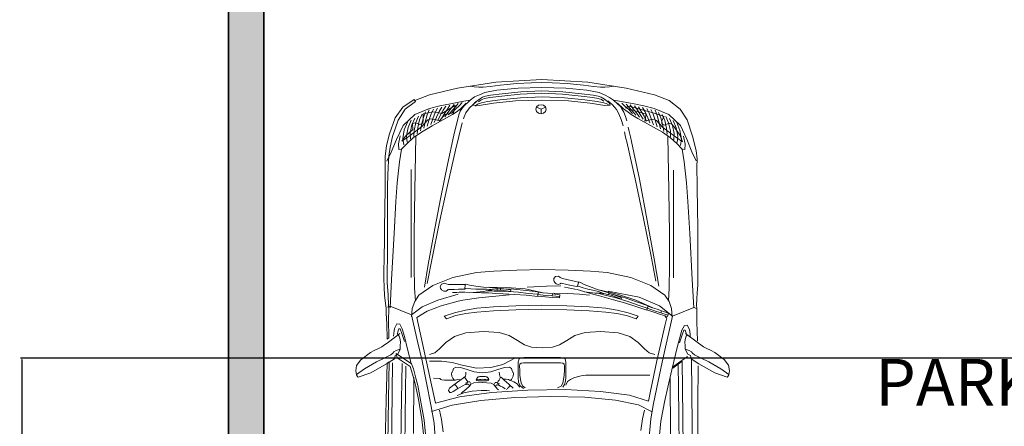
# Model space of a CAD drawing. Units: inches. Extents: x -5 to 366, y -496 to 54.
# Tile 2 of 10: x -5 to 121, y -389 to -337. Entities that reach past the tile are written whole.
import ezdxf

# ---------------------------------------------------------------- set-up
doc = ezdxf.new("R2010")
doc.units = ezdxf.units.IN
doc.header["$MEASUREMENT"] = 0
for name, color, linetype, lineweight in [('A-ANNO-DIMS', 2, 'Continuous', 18), ('A-AREA-IDEN', 7, 'Continuous', 25), ('A-SITE-VEHI', 8, 'Continuous', 13), ('A-WALL', 7, 'Continuous', 35), ('A-WALL-PATT', 252, 'Continuous', 13)]:
    doc.layers.add(name, color=color, linetype=linetype, lineweight=lineweight)
doc.styles.get("Standard").update_dxf_attribs({"font": 'arial.ttf'})
doc.dimstyles.get("Standard").update_dxf_attribs({"dimtxt": 0.18, "dimasz": 0.18, "dimexe": 0.18, "dimexo": 0.0625, "dimgap": 0.09, "dimtad": 0, "dimtih": 1, "dimtoh": 1, "dimdec": 0, "dimzin": 0, "dimdsep": 46, "dimlunit": 3, "dimtxsty": 'Standard', "dimcen": 0.09, "dimadec": 0, "dimazin": 0, "dimtfac": 1, "dimtdec": 0, "dimtofl": 0, "dimtmove": 0, "dimatfit": 3, "dimfxl": 1, "dimtolj": 1, "dimtzin": 0, "dimarcsym": 0})

# ---------------------------------------------------------------- blocks, each defined once
blk = doc.blocks.new('*D28')
at = {"layer": 'A-ANNO-DIMS', "color": 0, "lineweight": -2, "transparency": 16777216}
for p, q in [((165.37, -380.48), (-4.7, -380.48)), ((-4.52, -380.66), (-4.52, -398.3)), ((-4.52, -416.3), (-4.52, -398.66)), ((165.37, -416.48), (-4.7, -416.48))]:
    blk.add_line(p, q, dxfattribs=at)
at = {"layer": 'A-ANNO-DIMS', "color": 0, "transparency": 16777216}
for points in [[(-4.55, -380.66), (-4.49, -380.66), (-4.52, -380.48)], [(-4.55, -416.3), (-4.49, -416.3), (-4.52, -416.48)]]:
    blk.add_solid(points, dxfattribs=at)
at = {"layer": 'Defpoints', "color": 0, "transparency": 16777216}
for p in [(-4.52, -380.48), (165.43, -380.48), (165.43, -416.48)]:
    blk.add_point(p, dxfattribs=at)
at = {"layer": 'A-ANNO-DIMS', "color": 0, "transparency": 16777216, "insert": (-4.52, -398.48), "char_height": 0.18, "attachment_point": 5}
blk.add_mtext('\\A1;3\'-0"', dxfattribs=at)

msp = doc.modelspace()

# ---------------------------------------------------------------- hatches: boundary and pattern name
at = {"layer": 'A-WALL-PATT'}
h = msp.add_hatch(color=256, dxfattribs=at)
h.dxf.hatch_style = 1
h.paths.add_polyline_path([(324.93, 26.52), (21.93, 26.52), (21.93, -456.98), (26.43, -456.98), (26.43, -331.98), (30.93, -331.98), (30.93, -322.98), (30.93, -106.98), (110.93, -106.98), (110.93, -104.73), (110.93, -102.48), (30.93, -102.48), (30.93, 17.52), (138.93, 17.52), (141.18, 17.52), (143.43, 17.52), (183.43, 17.52), (187.93, 17.52), (315.93, 17.52), (315.93, -102.48), (315.93, -106.98), (315.93, -255.48), (171.93, -255.48), (171.93, -155.84), (167.43, -155.84), (167.43, -291.98), (171.93, -291.98), (171.93, -259.98), (315.93, -259.98), (315.93, -375.98), (297.93, -375.98), (297.93, -380.48), (315.93, -380.48), (315.93, -452.48), (315.93, -456.98), (324.93, -456.98)])
h.paths.add_polyline_path([(143.43, -18.48), (143.43, -13.98), (138.93, -13.98), (138.93, -106.98), (187.93, -106.98), (187.93, -102.48), (143.43, -102.48)], flags=17)

# ---------------------------------------------------------------- linework, layer by layer
at = {"layer": 'A-SITE-VEHI'}
for p, q in [((62.02, -344.83), (56.14, -345.18)), ((62.02, -344.83), (67.9, -345.18)), ((51.22, -345.93), (47.63, -346.8)), ((56.14, -345.18), (51.22, -345.93)), ((52.83, -345.68), (53.35, -345.78)), ((53.35, -345.78), (53.97, -345.81)), ((53.97, -345.81), (54.52, -345.79)), ((54.52, -345.79), (55.42, -345.7)), ((54.71, -346.48), (56.27, -346.18)), ((55.42, -345.7), (56.68, -345.56)), ((56.27, -346.18), (58.97, -345.93)), ((56.68, -345.56), (57.56, -345.45)), ((56.94, -346.64), (59.31, -346.41)), ((57.56, -345.45), (58.76, -345.35)), ((58.76, -345.35), (60.68, -345.26)), ((58.97, -345.93), (62.02, -345.83)), ((59.31, -346.41), (62.02, -346.29)), ((60.68, -345.26), (62.02, -345.21)), ((63.35, -345.26), (62.02, -345.21)), ((62.02, -345.83), (65.07, -345.93)), ((62.02, -346.29), (64.72, -346.41)), ((65.27, -345.35), (63.35, -345.26)), ((64.72, -346.41), (67.1, -346.64)), ((65.07, -345.93), (67.76, -346.18)), ((66.48, -345.45), (65.27, -345.35)), ((67.35, -345.56), (66.48, -345.45)), ((68.62, -345.7), (67.35, -345.56)), ((67.76, -346.18), (69.33, -346.48)), ((67.9, -345.18), (72.82, -345.93)), ((69.52, -345.79), (68.62, -345.7)), ((70.07, -345.81), (69.52, -345.79)), ((70.69, -345.78), (70.07, -345.81)), ((71.21, -345.68), (70.69, -345.78)), ((72.82, -345.93), (76.41, -346.8)), ((44.25, -348.36), (45.67, -347.39)), ((45.85, -347.66), (44.55, -348.62)), ((45.67, -347.39), (45.85, -347.66)), ((47.63, -346.8), (45.75, -347.52)), ((50.33, -347.93), (52.03, -347.6)), ((52.86, -347.45), (52.01, -348.26)), ((52.03, -347.6), (52.86, -347.45)), ((53.67, -347.64), (52.78, -348.46)), ((52.86, -347.45), (53.4, -347.06)), ((53.4, -347.06), (54.02, -346.77)), ((53.4, -347.8), (54.02, -347.33)), ((53.92, -347.7), (54.24, -347.42)), ((54.02, -346.77), (54.71, -346.48)), ((54.02, -347.33), (54.43, -347.08)), ((54.24, -347.42), (54.68, -347.25)), ((54.29, -347.79), (55.05, -347.65)), ((54.43, -347.08), (54.8, -346.94)), ((54.68, -347.25), (55.38, -347.13)), ((54.8, -346.94), (55.44, -346.83)), ((55.05, -347.65), (56.67, -347.44)), ((55.38, -347.13), (56.88, -346.94)), ((55.44, -346.83), (56.94, -346.64)), ((58.64, -347.57), (55.84, -347.86)), ((56.67, -347.44), (59.28, -347.17)), ((56.88, -346.94), (59.25, -346.7)), ((61.98, -347.45), (58.64, -347.57)), ((59.25, -346.7), (61.96, -346.59)), ((59.28, -347.17), (62.11, -347.03)), ((61.96, -346.59), (64.66, -346.7)), ((65.41, -347.57), (61.98, -347.45)), ((62.11, -347.03), (64.92, -347.17)), ((64.66, -346.7), (67.04, -346.94)), ((64.92, -347.17), (67.5, -347.44)), ((68.21, -347.86), (65.41, -347.57)), ((67.04, -346.94), (68.54, -347.13)), ((67.1, -346.64), (68.59, -346.83)), ((67.5, -347.44), (69.11, -347.65)), ((68.54, -347.13), (69.22, -347.24)), ((68.59, -346.83), (69.24, -346.94)), ((69.11, -347.65), (69.77, -347.76)), ((69.22, -347.24), (69.63, -347.39)), ((69.24, -346.94), (69.61, -347.08)), ((69.33, -346.48), (70.04, -346.8)), ((69.61, -347.08), (70.02, -347.33)), ((69.63, -347.39), (69.93, -347.61)), ((70.02, -347.33), (70.63, -347.8)), ((70.04, -346.8), (70.68, -347.12)), ((70.46, -347.55), (71, -348.04)), ((70.68, -347.12), (71.17, -347.45)), ((71.17, -347.45), (71.7, -347.94)), ((71.17, -347.45), (72.22, -347.63)), ((72.22, -347.63), (73.81, -347.94)), ((76.41, -346.8), (78.29, -347.52)), ((78.29, -347.52), (79.72, -348.6)), ((43.26, -349.71), (44.25, -348.36)), ((44.55, -348.62), (43.64, -350.03)), ((45.76, -349.32), (47.64, -348.55)), ((47.61, -348.71), (47.34, -349.36)), ((47.64, -348.55), (48.98, -348.21)), ((48.14, -348.6), (47.86, -349.21)), ((48.67, -348.48), (48.38, -349.06)), ((48.89, -348.91), (48.54, -349.66)), ((49.2, -348.36), (48.89, -348.91)), ((48.98, -348.21), (50.33, -347.93)), ((49.41, -348.77), (49.02, -349.45)), ((49.2, -349.17), (50.92, -348.17)), ((49.73, -348.25), (49.41, -348.77)), ((49.93, -348.62), (49.51, -349.24)), ((50.26, -348.13), (49.93, -348.62)), ((50.44, -348.47), (49.99, -349.04)), ((50.48, -348.83), (50.06, -349.35)), ((50.79, -348.02), (50.44, -348.47)), ((50.96, -348.32), (50.48, -348.83)), ((50.97, -348.62), (50.5, -349.1)), ((50.92, -348.17), (50.71, -349.08)), ((51.31, -347.9), (50.96, -348.32)), ((51.47, -348.17), (50.97, -348.62)), ((51.06, -349.01), (51.6, -348.57)), ((51.58, -348.86), (51.39, -349.34)), ((51.84, -347.78), (51.47, -348.17)), ((52.01, -348.26), (51.58, -348.86)), ((51.6, -348.57), (52.33, -347.87)), ((52.78, -348.46), (52.3, -349.1)), ((53.26, -348.13), (53.4, -347.8)), ((53.98, -348.14), (53.26, -348.13)), ((53.51, -348.23), (53.77, -347.98)), ((53.77, -347.98), (54.29, -347.79)), ((55.84, -347.86), (53.98, -348.14)), ((61.26, -348.63), (61.35, -348.34)), ((61.35, -348.92), (61.26, -348.63)), ((61.91, -348.63), (61.32, -348.38)), ((61.35, -348.34), (61.58, -348.13)), ((61.58, -349.12), (61.35, -348.92)), ((61.58, -348.13), (61.91, -348.05)), ((61.91, -348.05), (62.23, -348.13)), ((62.49, -348.38), (61.91, -348.63)), ((61.91, -348.63), (61.91, -349.2)), ((62.23, -348.13), (62.47, -348.34)), ((62.47, -348.92), (62.23, -349.12)), ((62.47, -348.34), (62.56, -348.63)), ((62.56, -348.63), (62.47, -348.92)), ((70.06, -348.14), (68.21, -347.86)), ((69.77, -347.76), (70.23, -347.89)), ((70.77, -348.13), (70.06, -348.14)), ((70.23, -347.89), (70.62, -348.1)), ((70.63, -347.8), (70.77, -348.13)), ((71, -348.04), (71.36, -348.39)), ((71.36, -348.39), (71.56, -348.65)), ((71.56, -348.65), (71.85, -349.2)), ((71.7, -347.94), (72.06, -348.3)), ((72.48, -348.57), (71.71, -347.87)), ((72.06, -348.3), (72.25, -348.56)), ((72.25, -348.56), (72.49, -349.02)), ((72.27, -347.84), (72.64, -348.23)), ((73.08, -349), (72.48, -348.57)), ((72.64, -348.23), (73.15, -348.68)), ((73.19, -348.23), (72.72, -348.44)), ((72.72, -348.44), (75.38, -349.25)), ((72.8, -347.96), (73.16, -348.38)), ((73.15, -348.68), (73.61, -349.16)), ((73.16, -348.38), (73.63, -348.89)), ((75.15, -348.8), (73.19, -348.23)), ((73.33, -348.07), (73.67, -348.53)), ((73.63, -348.89), (74.06, -349.4)), ((73.67, -348.53), (74.12, -349.09)), ((73.81, -347.94), (75.06, -348.21)), ((73.86, -348.19), (74.19, -348.68)), ((74.19, -348.68), (74.61, -349.3)), ((74.38, -348.31), (74.7, -348.83)), ((74.7, -348.83), (75.09, -349.51)), ((74.91, -348.42), (75.22, -348.97)), ((75.06, -348.21), (76.4, -348.55)), ((75.5, -348.89), (75.15, -348.8)), ((75.44, -348.54), (75.74, -349.12)), ((76.4, -349.14), (75.5, -348.89)), ((75.97, -348.66), (76.25, -349.27)), ((76.4, -348.55), (78.28, -349.32)), ((76.5, -348.77), (76.77, -349.42)), ((79.72, -348.6), (80.61, -350)), ((42.52, -351.77), (43.26, -349.71)), ((43.64, -350.03), (42.92, -352.11)), ((44.29, -350.71), (45.76, -349.32)), ((45.3, -350.02), (44.91, -350.96)), ((45.76, -349.76), (45.39, -350.64)), ((46.23, -349.5), (45.88, -350.32)), ((46.37, -350), (46.13, -350.98)), ((46.69, -349.24), (46.37, -350)), ((46.86, -349.68), (46.6, -350.64)), ((47.41, -350), (46.61, -350.89)), ((46.77, -350.42), (46.85, -349.96)), ((46.83, -349.23), (48.06, -348.98)), ((46.85, -349.46), (46.83, -349.23)), ((46.85, -349.96), (46.85, -349.46)), ((47.15, -348.98), (46.86, -349.68)), ((47.34, -349.36), (47.08, -350.29)), ((47.56, -350.08), (47.36, -350.81)), ((47.75, -349.84), (47.41, -350)), ((47.86, -349.21), (47.56, -350.08)), ((48.49, -349.98), (47.75, -349.84)), ((48.05, -349.87), (47.81, -350.57)), ((47.97, -350.75), (49.42, -349.94)), ((48.38, -349.06), (48.05, -349.87)), ((48.06, -348.98), (48.89, -349.07)), ((48.54, -349.66), (48.26, -350.32)), ((48.91, -350.1), (48.49, -349.98)), ((49.02, -349.45), (48.71, -350.08)), ((48.89, -349.07), (49.2, -349.17)), ((49.62, -349.29), (48.91, -350.1)), ((49.51, -349.24), (49.16, -349.83)), ((49.42, -349.94), (50.6, -349.29)), ((49.99, -349.04), (49.61, -349.59)), ((50.71, -349.08), (49.62, -349.29)), ((50.6, -349.29), (51.06, -349.01)), ((51.39, -349.34), (50.74, -351.93)), ((52.08, -349.61), (52.01, -349.84)), ((52.3, -349.1), (52.08, -349.61)), ((61.91, -349.2), (61.58, -349.12)), ((62.23, -349.12), (61.91, -349.2)), ((71.85, -349.2), (72.16, -349.94)), ((72.16, -349.94), (72.4, -350.76)), ((72.49, -349.02), (72.7, -349.55)), ((72.7, -349.55), (72.89, -350.13)), ((73.44, -349.29), (73.08, -349)), ((74.31, -349.83), (73.44, -349.29)), ((74.12, -349.09), (74.51, -349.65)), ((75.91, -350.69), (74.31, -349.83)), ((74.61, -349.3), (74.96, -349.89)), ((75.09, -349.51), (75.41, -350.14)), ((75.38, -349.25), (75.21, -350.16)), ((75.21, -350.16), (75.62, -350.04)), ((75.22, -348.97), (75.58, -349.72)), ((75.58, -349.72), (75.85, -350.38)), ((75.62, -350.04), (76.37, -349.9)), ((75.74, -349.12), (76.06, -349.93)), ((76.06, -349.93), (76.3, -350.63)), ((76.25, -349.27), (76.55, -350.14)), ((76.37, -349.9), (76.7, -350.06)), ((77.66, -349.57), (76.4, -349.14)), ((76.55, -350.14), (76.75, -350.87)), ((76.7, -350.06), (77.5, -350.95)), ((76.77, -349.42), (77.04, -350.35)), ((76.96, -349.03), (77.26, -349.74)), ((77.26, -349.74), (77.51, -350.7)), ((77.35, -350.48), (77.36, -350.1)), ((77.36, -350.1), (77.54, -349.73)), ((77.42, -349.3), (77.74, -350.06)), ((77.54, -349.73), (77.66, -349.57)), ((77.74, -350.06), (77.98, -351.04)), ((77.89, -349.56), (78.23, -350.38)), ((78.28, -349.32), (79.75, -350.71)), ((78.35, -349.82), (78.72, -350.7)), ((78.81, -350.08), (79.21, -351.02)), ((80.61, -350), (81.29, -352.06)), ((43.43, -352.5), (44.29, -350.71)), ((44.42, -351.28), (44.24, -352.37)), ((44.84, -350.28), (44.42, -351.28)), ((44.59, -352.06), (45.5, -351.22)), ((44.91, -350.96), (44.71, -352.03)), ((46.61, -350.89), (45, -352.11)), ((45.39, -350.64), (45.18, -351.68)), ((45.47, -350.47), (45.84, -350.37)), ((45.5, -351.22), (45.47, -350.47)), ((45.66, -351.33), (45.63, -352.12)), ((45.88, -350.32), (45.66, -351.33)), ((45.84, -350.37), (46.41, -350.6)), ((46.13, -350.98), (46.05, -351.77)), ((46.41, -350.6), (46.77, -350.42)), ((46.6, -350.64), (46.48, -351.41)), ((46.6, -351.56), (47.97, -350.75)), ((47.08, -350.29), (46.91, -351.06)), ((51.84, -350.39), (50.95, -353.85)), ((73.05, -350.91), (73.19, -351.48)), ((77.44, -351.56), (75.91, -350.69)), ((77.04, -350.35), (77.2, -351.12)), ((77.71, -350.66), (77.35, -350.48)), ((77.5, -350.95), (79.11, -352.17)), ((77.51, -350.7), (77.63, -351.47)), ((78.28, -350.43), (77.71, -350.66)), ((77.98, -351.04), (78.06, -351.83)), ((78.23, -350.38), (78.46, -351.39)), ((78.65, -350.53), (78.28, -350.43)), ((78.46, -351.39), (78.49, -352.18)), ((79.04, -351), (78.65, -350.53)), ((78.72, -350.7), (78.93, -351.74)), ((79.73, -351.98), (79.04, -351)), ((79.21, -351.02), (79.4, -352.09)), ((79.28, -350.34), (79.69, -351.34)), ((79.69, -351.34), (79.88, -352.43)), ((79.75, -350.71), (80.58, -352.48)), ((42.15, -353.29), (42.52, -351.77)), ((42.92, -352.11), (42.59, -353.49)), ((42.75, -354.12), (43.43, -352.5)), ((43.89, -352.03), (43.68, -353.07)), ((44.12, -352.73), (44.59, -352.06)), ((45, -352.11), (44.12, -352.73)), ((44.24, -352.37), (44.34, -353.19)), ((44.71, -352.03), (44.77, -352.83)), ((44.77, -353.01), (45.55, -352.3)), ((45.18, -351.68), (45.2, -352.48)), ((45.55, -352.3), (46.6, -351.56)), ((45.9, -352.06), (45.77, -359.02)), ((50.74, -351.93), (49.93, -355.71)), ((72.57, -351.54), (72.67, -351.97)), ((72.67, -351.97), (72.77, -352.39)), ((72.77, -352.39), (72.87, -352.82)), ((73.19, -351.48), (73.35, -352.18)), ((73.35, -352.18), (73.49, -352.75)), ((78.48, -352.3), (77.44, -351.56)), ((78.13, -352.06), (78.26, -359.02)), ((79.27, -353.01), (78.48, -352.3)), ((78.93, -351.74), (78.92, -352.54)), ((79.11, -352.17), (79.99, -352.78)), ((79.4, -352.09), (79.34, -352.89)), ((79.99, -352.78), (79.73, -351.98)), ((79.88, -352.43), (79.77, -353.25)), ((80.16, -352.07), (80.36, -353.09)), ((80.58, -352.48), (81.22, -354.07)), ((81.29, -352.06), (81.75, -353.93)), ((41.97, -354.69), (42.15, -353.29)), ((42.59, -353.49), (42.44, -354.64)), ((43.68, -353.07), (43.71, -353.79)), ((43.71, -353.79), (44.06, -353.75)), ((44.06, -353.75), (43.82, -355.34)), ((44.06, -353.75), (44.77, -353.01)), ((50.95, -353.85), (49.93, -358.39)), ((72.87, -352.82), (73.94, -357.53)), ((73.49, -352.75), (74.49, -357.58)), ((79.98, -353.75), (79.27, -353.01)), ((79.98, -353.75), (80.22, -355.34)), ((80.32, -353.79), (79.98, -353.75)), ((80.36, -353.09), (80.32, -353.79)), ((81.75, -353.93), (81.89, -355.02)), ((41.96, -356.21), (41.97, -354.69)), ((42.17, -355.29), (42.75, -354.12)), ((42.44, -354.64), (42.35, -356.02)), ((81.22, -354.07), (81.76, -355.22)), ((81.89, -355.02), (81.86, -356.02)), ((41.95, -358.51), (41.96, -356.21)), ((42.35, -356.02), (42.29, -358.36)), ((43.82, -355.34), (43.52, -358.03)), ((45.3, -370.15), (45.3, -356.32)), ((49.93, -355.71), (49.05, -360.1)), ((78.84, -370.19), (78.84, -356.42)), ((80.22, -355.34), (80.52, -358.03)), ((81.86, -356.02), (81.88, -358.37)), ((73.94, -357.53), (75.02, -362.59)), ((74.49, -357.58), (75.5, -362.88)), ((41.91, -361.65), (41.95, -358.51)), ((42.29, -358.36), (42.26, -361.6)), ((43.52, -358.03), (43.33, -360.45)), ((49.93, -358.39), (48.9, -363.25)), ((80.52, -358.03), (80.71, -360.45)), ((81.88, -358.37), (81.94, -361.6)), ((45.77, -359.02), (45.7, -364.54)), ((49.05, -360.1), (48.21, -364.56)), ((78.26, -359.02), (78.33, -364.54)), ((43.33, -360.45), (43.11, -364.53)), ((80.71, -360.45), (80.93, -364.53)), ((41.88, -363.56), (41.91, -361.65)), ((42.26, -361.6), (42.25, -363.56)), ((75.02, -362.59), (75.96, -367.23)), ((81.94, -361.6), (81.98, -363.56)), ((41.87, -365.2), (41.88, -363.56)), ((42.25, -363.56), (42.25, -365.19)), ((48.9, -363.25), (47.99, -367.68)), ((75.5, -362.88), (76.38, -367.75)), ((81.98, -363.56), (81.97, -365.15)), ((41.85, -367.71), (41.87, -365.2)), ((42.25, -365.19), (42.25, -367.69)), ((43.11, -364.53), (42.78, -370.42)), ((45.7, -364.54), (45.69, -368.69)), ((48.21, -364.56), (47.49, -368.51)), ((78.33, -364.54), (78.34, -368.69)), ((80.93, -364.53), (81.25, -370.42)), ((81.97, -365.15), (81.96, -367.57)), ((41.82, -369.33), (41.85, -367.71)), ((42.25, -367.69), (42.22, -369.3)), ((47.99, -367.68), (47.35, -370.93)), ((75.96, -367.23), (76.61, -370.64)), ((76.38, -367.75), (76.98, -371.27)), ((81.96, -367.57), (81.98, -369.14)), ((45.69, -368.69), (45.73, -371.53)), ((47.49, -368.51), (47, -371.39)), ((78.34, -368.69), (78.3, -371.53)), ((41.8, -370.23), (41.82, -369.33)), ((41.83, -371.43), (41.8, -370.23)), ((42.22, -369.3), (42.22, -370.83)), ((50.63, -370.15), (48.07, -371.17)), ((53.65, -369.52), (50.63, -370.15)), ((55.86, -369.35), (53.65, -369.52)), ((58.8, -369.24), (55.86, -369.35)), ((62.12, -369.15), (58.8, -369.24)), ((65.39, -369.24), (62.12, -369.15)), ((63.56, -370.53), (63.57, -370.29)), ((63.57, -370.29), (63.77, -370.03)), ((63.77, -370.03), (64.16, -369.99)), ((64.16, -369.99), (64.38, -370.14)), ((64.38, -370.14), (64.64, -370.28)), ((64.64, -370.28), (66.71, -370.75)), ((68.23, -369.35), (65.39, -369.24)), ((70.38, -369.52), (68.23, -369.35)), ((73.41, -370.15), (70.38, -369.52)), ((75.97, -371.17), (73.41, -370.15)), ((81.99, -370.01), (81.97, -371.15)), ((81.98, -369.14), (81.99, -370.01)), ((41.9, -372.41), (41.83, -371.43)), ((42.22, -370.83), (42.34, -372.32)), ((42.78, -370.42), (42.6, -374.02)), ((45.73, -371.53), (45.83, -373.14)), ((48.07, -371.17), (46.29, -372.44)), ((49.02, -371.3), (49.16, -371.01)), ((49.07, -371.55), (49.02, -371.3)), ((49.16, -371.69), (49.07, -371.55)), ((49.16, -371.01), (49.53, -370.88)), ((49.53, -370.88), (49.78, -370.98)), ((49.78, -370.98), (50.07, -371.05)), ((50.07, -371.05), (52.19, -371.04)), ((52.19, -371.01), (52.16, -371.68)), ((52.47, -371.06), (52.19, -371.01)), ((52.91, -371.61), (52.25, -371.57)), ((52.76, -371.13), (52.47, -371.06)), ((53.03, -371.18), (52.76, -371.13)), ((53.55, -371.65), (52.91, -371.61)), ((53.89, -371.3), (53.03, -371.18)), ((54.53, -371.38), (53.89, -371.3)), ((55.33, -371.45), (54.53, -371.38)), ((57.51, -371.43), (55.14, -371.41)), ((55.65, -371.48), (55.33, -371.45)), ((55.98, -371.51), (55.65, -371.48)), ((56.29, -371.53), (55.98, -371.51)), ((56.3, -371.55), (56.28, -371.79)), ((56.87, -371.58), (56.29, -371.54)), ((56.74, -371.57), (56.72, -371.78)), ((57.46, -371.65), (56.87, -371.58)), ((56.91, -371.6), (58.45, -371.67)), ((59.87, -371.63), (57.51, -371.43)), ((60.99, -371.36), (60.14, -371.41)), ((62.59, -371.27), (60.99, -371.36)), ((64.44, -371.22), (62.59, -371.27)), ((63.61, -370.69), (63.56, -370.53)), ((63.67, -370.8), (63.61, -370.69)), ((63.86, -370.98), (63.67, -370.8)), ((64.16, -371.05), (63.86, -370.98)), ((64.37, -370.98), (64.16, -371.05)), ((64.4, -370.92), (64.37, -370.98)), ((64.44, -370.89), (64.4, -370.92)), ((65.22, -371.05), (64.5, -370.9)), ((64.93, -371.4), (65.38, -371.5)), ((65.76, -371.17), (65.22, -371.05)), ((65.38, -371.5), (66.01, -371.62)), ((66.48, -371.32), (65.76, -371.17)), ((66.73, -370.71), (66.54, -371.36)), ((67.29, -371.46), (66.66, -371.27)), ((67.05, -370.86), (66.73, -370.71)), ((67.45, -371.06), (67.05, -370.86)), ((67.9, -371.65), (67.29, -371.46)), ((67.78, -371.2), (67.45, -371.06)), ((68.44, -371.42), (67.78, -371.2)), ((69.01, -371.64), (68.44, -371.42)), ((77.75, -372.44), (75.97, -371.17)), ((78.3, -371.53), (78.21, -373.14)), ((81.25, -370.42), (81.44, -374.02)), ((81.97, -371.15), (81.9, -372.1)), ((41.98, -373.14), (41.9, -372.41)), ((42.34, -372.32), (42.4, -373.84)), ((46.29, -372.44), (45.75, -373.21)), ((51.31, -372.31), (48.69, -373.04)), ((49.24, -371.78), (49.16, -371.69)), ((49.46, -371.92), (49.24, -371.78)), ((49.77, -371.91), (49.46, -371.92)), ((49.96, -371.8), (49.77, -371.91)), ((49.98, -371.73), (49.96, -371.8)), ((50.01, -371.69), (49.98, -371.73)), ((50.8, -371.68), (50.07, -371.69)), ((50.6, -372.08), (50.87, -372.08)), ((51.35, -371.67), (50.8, -371.68)), ((50.87, -372.08), (51.15, -372.07)), ((51.15, -372.07), (51.42, -372.05)), ((52.09, -371.66), (51.35, -371.67)), ((51.42, -372.05), (51.67, -372.05)), ((51.67, -372.05), (51.91, -372.04)), ((51.91, -372.04), (52.15, -372.03)), ((53.96, -372.74), (51.91, -373.06)), ((52.25, -372.02), (54.3, -372.13)), ((53.23, -372.07), (54.56, -371.94)), ((54.22, -371.66), (53.55, -371.65)), ((57.85, -372.39), (53.96, -372.74)), ((54.95, -371.66), (54.22, -371.66)), ((54.3, -372.13), (55.21, -372.14)), ((54.93, -371.87), (54.56, -371.94)), ((55.86, -371.9), (54.91, -371.87)), ((55.3, -371.8), (54.93, -371.87)), ((55.54, -371.71), (54.95, -371.66)), ((55.21, -372.14), (56.13, -372.19)), ((55.68, -371.77), (55.3, -371.8)), ((56.28, -371.79), (55.54, -371.71)), ((56.81, -371.91), (55.86, -371.9)), ((56.13, -372.19), (57.05, -372.24)), ((56.27, -371.75), (56.85, -371.79)), ((57.76, -371.95), (56.81, -371.91)), ((56.85, -371.79), (57.44, -371.85)), ((57.05, -372.24), (58.53, -372.32)), ((57.44, -371.85), (58.02, -371.93)), ((58.04, -371.74), (57.46, -371.65)), ((59.01, -372.05), (57.76, -371.95)), ((58.04, -371.74), (58.01, -371.93)), ((58.45, -371.67), (59.99, -371.83)), ((58.53, -372.32), (60.03, -372.42)), ((60.26, -372.19), (59.01, -372.05)), ((62.18, -372.1), (59.87, -371.63)), ((59.99, -371.83), (61.53, -372)), ((60.03, -372.42), (61.5, -372.59)), ((61.51, -372.31), (60.26, -372.19)), ((61.53, -372), (61.5, -372.54)), ((62.51, -372.45), (61.5, -372.33)), ((61.5, -372.54), (62.42, -372.64)), ((61.53, -372.04), (62.14, -372.11)), ((62.14, -372.11), (62.75, -372.16)), ((62.42, -372.64), (63.35, -372.71)), ((62.51, -372.45), (63.34, -372.52)), ((62.75, -372.16), (63.36, -372.22)), ((63.36, -372.24), (63.34, -372.52)), ((63.34, -372.52), (64.28, -372.59)), ((63.35, -372.71), (64.28, -372.76)), ((63.36, -372.24), (63.67, -372.28)), ((65.3, -372.19), (63.57, -372.16)), ((63.67, -372.28), (63.99, -372.32)), ((63.99, -372.32), (64.3, -372.36)), ((64.3, -372.36), (64.28, -372.76)), ((66.82, -372.28), (65.3, -372.19)), ((66.01, -371.62), (66.45, -371.7)), ((66.55, -371.71), (68.52, -372.28)), ((68.11, -372.4), (66.82, -372.28)), ((67.49, -371.98), (68.82, -372.15)), ((68.55, -371.8), (67.9, -371.65)), ((68.52, -372.28), (69.41, -372.5)), ((69.26, -371.97), (68.55, -371.8)), ((69.2, -372.17), (68.82, -372.15)), ((69.68, -371.85), (69.01, -371.64)), ((70.09, -372.41), (69.17, -372.17)), ((69.58, -372.18), (69.2, -372.17)), ((69.82, -372.15), (69.26, -371.97)), ((69.41, -372.5), (70.3, -372.75)), ((71.81, -372.32), (69.51, -371.76)), ((69.95, -372.24), (69.58, -372.18)), ((69.99, -371.94), (69.68, -371.85)), ((70.53, -372.39), (69.82, -372.15)), ((70.3, -372.05), (69.99, -371.94)), ((71.02, -372.63), (70.09, -372.41)), ((70.6, -372.14), (70.3, -372.05)), ((70.3, -372.75), (71.18, -373.01)), ((74.46, -372.66), (70.5, -371.89)), ((70.6, -372.17), (70.53, -372.39)), ((70.53, -372.35), (71.09, -372.52)), ((71.15, -372.32), (70.59, -372.15)), ((71.02, -372.28), (70.96, -372.48)), ((71.93, -372.88), (71.02, -372.63)), ((71.09, -372.52), (71.65, -372.72)), ((71.71, -372.53), (71.15, -372.32)), ((71.19, -372.35), (72.67, -372.76)), ((71.65, -372.72), (72.19, -372.92)), ((72.26, -372.74), (71.71, -372.53)), ((74.06, -373.05), (71.81, -372.32)), ((72.26, -372.74), (72.18, -372.92)), ((72.67, -372.76), (74.14, -373.27)), ((77.08, -373.79), (74.46, -372.66)), ((78.29, -373.21), (77.75, -372.44)), ((81.9, -372.1), (81.84, -372.9)), ((42.04, -373.77), (41.98, -373.14)), ((42.08, -374.1), (42.04, -373.77)), ((42.11, -374.76), (42.08, -374.1)), ((42.25, -373.95), (42.63, -373.84)), ((42.4, -373.84), (42.42, -373.87)), ((42.42, -373.87), (42.42, -373.91)), ((42.42, -373.91), (42.43, -373.95)), ((42.43, -373.95), (42.42, -374.29)), ((42.63, -373.84), (45.35, -374.95)), ((46.7, -373.93), (45.35, -374.95)), ((45.75, -373.21), (45.44, -374.14)), ((48.69, -373.04), (46.7, -373.93)), ((49.13, -373.78), (47.36, -374.47)), ((51.31, -373.2), (49.13, -373.78)), ((51.91, -373.06), (51.31, -373.2)), ((53.69, -374.08), (52.23, -374.32)), ((55.84, -373.91), (53.69, -374.08)), ((58.68, -373.8), (55.84, -373.91)), ((61.95, -373.72), (58.68, -373.8)), ((65.21, -373.8), (61.95, -373.72)), ((68.06, -373.91), (65.21, -373.8)), ((70.21, -374.08), (68.06, -373.91)), ((71.67, -374.32), (70.21, -374.08)), ((71.18, -373.01), (72.6, -373.42)), ((73.13, -373.27), (71.93, -372.88)), ((72.6, -373.42), (74.04, -373.85)), ((74.32, -373.68), (73.13, -373.27)), ((74.04, -373.85), (75.43, -374.34)), ((76.21, -374.03), (74.06, -373.05)), ((74.14, -373.27), (75.6, -373.78)), ((75.51, -374.08), (74.32, -373.68)), ((75.6, -373.78), (75.44, -374.3)), ((76.45, -374.44), (75.5, -374.09)), ((75.58, -373.82), (76.16, -374.02)), ((76.16, -374.02), (76.75, -374.21)), ((78.73, -375.11), (77.08, -373.79)), ((78.6, -374.14), (78.29, -373.21)), ((81.44, -374), (78.73, -375.11)), ((81.82, -374.12), (81.44, -374)), ((81.84, -372.9), (81.81, -373.69)), ((81.81, -373.69), (81.83, -374.14)), ((42.17, -376.09), (42.11, -374.76)), ((42.42, -374.29), (42.41, -375.5)), ((45.35, -374.95), (45.61, -376.08)), ((45.44, -374.14), (45.36, -375.18)), ((47.36, -374.47), (46.01, -375.26)), ((46.01, -375.26), (48.42, -386.25)), ((50.83, -374.66), (49.54, -375.09)), ((49.54, -375.09), (49.8, -375.43)), ((49.8, -375.43), (51.03, -375.04)), ((52.23, -374.32), (50.83, -374.66)), ((51.03, -375.04), (52.3, -374.78)), ((52.3, -374.78), (53.69, -374.59)), ((53.69, -374.59), (55.84, -374.42)), ((55.84, -374.42), (58.68, -374.3)), ((58.68, -374.3), (61.95, -374.22)), ((61.95, -374.22), (65.21, -374.3)), ((65.21, -374.3), (68.06, -374.42)), ((68.06, -374.42), (70.21, -374.59)), ((70.21, -374.59), (71.6, -374.78)), ((71.6, -374.78), (72.86, -375.04)), ((73.06, -374.66), (71.67, -374.32)), ((72.86, -375.04), (74.09, -375.43)), ((74.35, -375.09), (73.06, -374.66)), ((74.09, -375.43), (74.35, -375.09)), ((75.44, -374.3), (76.33, -374.61)), ((76.33, -374.61), (77.21, -374.89)), ((76.45, -374.44), (77.24, -374.69)), ((76.75, -374.21), (77.33, -374.41)), ((77.21, -374.89), (78.11, -375.14)), ((77.33, -374.43), (77.24, -374.69)), ((77.24, -374.69), (78.15, -374.97)), ((77.33, -374.43), (77.63, -374.53)), ((77.63, -374.53), (77.92, -374.64)), ((77.82, -375.19), (77.73, -375.13)), ((77.76, -376.36), (78, -375.33)), ((77.91, -375.26), (77.82, -375.19)), ((78, -375.33), (77.91, -375.26)), ((77.92, -374.64), (78.22, -374.75)), ((78.22, -374.75), (78.11, -375.14)), ((78.73, -375.11), (78.47, -376.25)), ((78.67, -375.18), (78.6, -374.14)), ((81.83, -374.14), (81.83, -374.55)), ((81.83, -374.55), (81.86, -375.89)), ((42.22, -378.04), (42.17, -376.09)), ((42.41, -375.5), (42.43, -377.86)), ((43.17, -376.67), (43.48, -376.08)), ((43.48, -376.08), (43.83, -376.13)), ((43.83, -376.13), (44.16, -376.74)), ((45.61, -376.08), (46.17, -378.53)), ((77.23, -378.61), (77.76, -376.36)), ((78.47, -376.25), (77.91, -378.69)), ((80.25, -376.29), (79.91, -376.91)), ((80.6, -376.25), (80.25, -376.29)), ((80.91, -376.83), (80.6, -376.25)), ((81.86, -375.89), (81.93, -378.25)), ((42.43, -377.86), (42.22, -378.04)), ((43.84, -377.33), (42.38, -378.42)), ((43.08, -377.33), (43.05, -377.66)), ((43.12, -376.99), (43.08, -377.33)), ((43.17, -376.67), (43.12, -376.99)), ((43.53, -377.35), (43.51, -377.43)), ((43.59, -377.11), (43.53, -377.35)), ((43.7, -376.74), (43.59, -377.11)), ((43.69, -377.59), (43.75, -377.68)), ((43.88, -376.72), (43.7, -376.74)), ((43.75, -377.68), (43.86, -377.93)), ((44.12, -377.33), (43.88, -376.72)), ((44.43, -378.35), (44.12, -377.33)), ((44.16, -376.74), (44.44, -377.72)), ((44.44, -377.72), (44.84, -379.33)), ((49.73, -378.46), (50.82, -377.7)), ((50.82, -377.7), (52.3, -377.24)), ((52.3, -377.24), (54.56, -377.08)), ((54.56, -377.08), (56.54, -377.21)), ((56.54, -377.21), (57.83, -377.59)), ((57.83, -377.59), (58.88, -378.2)), ((65.2, -378.2), (66.25, -377.59)), ((66.25, -377.59), (67.54, -377.21)), ((67.54, -377.21), (69.52, -377.08)), ((69.52, -377.08), (71.78, -377.24)), ((71.78, -377.24), (73.26, -377.7)), ((73.26, -377.7), (74.35, -378.46)), ((79.91, -376.91), (79.37, -378.93)), ((79.64, -378.51), (79.95, -377.49)), ((79.95, -377.49), (80.19, -376.88)), ((80.19, -376.88), (80.37, -376.91)), ((80.37, -376.91), (80.49, -377.27)), ((80.5, -377.68), (80.39, -377.93)), ((80.41, -377.33), (81.87, -378.42)), ((80.49, -377.27), (80.55, -377.51)), ((80.56, -377.59), (80.5, -377.68)), ((80.55, -377.51), (80.56, -377.59)), ((80.91, -376.83), (80.95, -377.11)), ((80.95, -377.11), (80.98, -377.4)), ((80.98, -377.4), (81.01, -377.69)), ((41.55, -379.05), (41.22, -379.2)), ((41.71, -378.92), (41.55, -379.05)), ((42.38, -378.42), (41.71, -378.92)), ((43.86, -377.93), (43.92, -378.4)), ((43.91, -378.89), (43.89, -379.2)), ((43.92, -378.4), (43.91, -378.89)), ((46.17, -378.53), (46.69, -380.83)), ((48.92, -379.27), (49.73, -378.46)), ((58.88, -378.2), (59.79, -378.76)), ((59.79, -378.76), (60.68, -379.06)), ((60.68, -379.06), (62.04, -379.14)), ((62.04, -379.14), (63.4, -379.06)), ((63.4, -379.06), (64.29, -378.76)), ((64.29, -378.76), (65.2, -378.2)), ((74.35, -378.46), (75.16, -379.27)), ((76.74, -380.82), (77.23, -378.61)), ((77.91, -378.69), (77.39, -381)), ((79.37, -378.93), (78.63, -381.99)), ((80.39, -377.93), (80.33, -378.4)), ((80.33, -378.4), (80.34, -378.89)), ((80.34, -378.89), (80.36, -379.2)), ((81.87, -378.42), (82.54, -378.92)), ((82.54, -378.92), (82.7, -379.05)), ((82.7, -379.05), (83.03, -379.2)), ((40.1, -379.77), (38.84, -380.68)), ((40.58, -379.52), (40.1, -379.77)), ((41.22, -379.2), (40.58, -379.52)), ((42.26, -380.27), (41.85, -380.46)), ((42.71, -380.04), (42.26, -380.27)), ((42.96, -379.85), (42.71, -380.04)), ((43.1, -379.69), (42.96, -379.85)), ((43.39, -379.5), (43.1, -379.69)), ((43.15, -380.58), (43.23, -380.12)), ((43.57, -379.96), (43.23, -380.12)), ((43.88, -379.31), (43.39, -379.5)), ((43.39, -379.89), (45.33, -381.19)), ((43.52, -380.42), (43.39, -379.89)), ((45.15, -381.56), (43.52, -380.42)), ((43.88, -379.31), (43.57, -379.96)), ((43.89, -379.2), (43.88, -379.31)), ((44.84, -379.33), (45.29, -381.17)), ((47.63, -379.99), (48.33, -379.8)), ((48.33, -379.8), (48.92, -379.27)), ((59.84, -380.4), (58.57, -380.5)), ((59.35, -380.42), (59.1, -380.57)), ((59.69, -380.4), (59.35, -380.42)), ((64.39, -380.4), (59.69, -380.4)), ((62.39, -380.41), (59.84, -380.4)), ((66.25, -380.42), (62.39, -380.41)), ((64.74, -380.42), (64.39, -380.4)), ((64.98, -380.57), (64.74, -380.42)), ((71.04, -380.42), (66.25, -380.42)), ((76.36, -380.41), (71.04, -380.42)), ((75.16, -379.27), (75.75, -379.8)), ((75.75, -379.8), (76.46, -379.99)), ((80.64, -380.27), (78.77, -381.61)), ((80.36, -379.2), (80.37, -379.31)), ((80.37, -379.31), (80.68, -379.96)), ((80.37, -379.31), (80.86, -379.5)), ((80.68, -379.96), (81.02, -380.12)), ((80.86, -379.5), (81.15, -379.69)), ((81.1, -380.58), (81.02, -380.12)), ((81.15, -379.69), (81.29, -379.85)), ((81.29, -379.85), (81.54, -380.04)), ((81.54, -380.04), (81.99, -380.27)), ((81.99, -380.27), (82.4, -380.46)), ((83.03, -379.2), (83.68, -379.52)), ((83.68, -379.52), (84.16, -379.77)), ((84.16, -379.77), (85.33, -380.64)), ((38.31, -381.42), (38.22, -382.09)), ((38.84, -380.68), (38.31, -381.42)), ((40.88, -380.97), (39.32, -381.84)), ((40.12, -382.35), (42.15, -381.2)), ((41.85, -380.46), (40.88, -380.97)), ((42.1, -385.84), (42.22, -381.12)), ((42.15, -381.2), (43.15, -380.58)), ((42.22, -381.12), (42.5, -380.95)), ((42.5, -380.95), (42.39, -385.7)), ((42.9, -381.09), (42.89, -382.31)), ((44.13, -381.18), (44.03, -388.16)), ((44.6, -381.51), (44.51, -387.97)), ((45.47, -382.52), (45.15, -381.56)), ((45.33, -381.19), (45.59, -381.85)), ((46.69, -380.83), (47.23, -383.44)), ((49.16, -380.85), (47.63, -380.85)), ((50.56, -381.03), (49.16, -380.85)), ((51.82, -381.39), (50.56, -381.03)), ((50.73, -381.8), (51, -381.65)), ((51, -381.65), (51.62, -381.69)), ((51.62, -381.69), (52.47, -381.93)), ((53.65, -381.76), (51.82, -381.39)), ((55.5, -381.67), (53.65, -381.76)), ((57.03, -381.27), (55.5, -381.67)), ((57.24, -381.69), (56.4, -381.93)), ((57.92, -380.81), (57.03, -381.27)), ((57.86, -381.65), (57.24, -381.69)), ((58.13, -381.8), (57.86, -381.65)), ((58.57, -380.5), (57.92, -380.81)), ((59.1, -380.57), (59, -381.01)), ((59, -381.01), (59, -382.94)), ((59.21, -381.26), (59.17, -381.51)), ((59.17, -381.51), (59.18, -382)), ((59.36, -381.13), (59.21, -381.26)), ((59.67, -381.09), (59.36, -381.13)), ((59.67, -381.09), (64.41, -381.09)), ((64.41, -381.09), (64.72, -381.13)), ((64.72, -381.13), (64.87, -381.26)), ((64.87, -381.26), (64.91, -381.51)), ((64.91, -381.51), (64.9, -382)), ((65.08, -381.01), (64.98, -380.57)), ((65.08, -382.94), (65.08, -381.01)), ((76.35, -382.67), (76.74, -380.82)), ((77.39, -381), (76.88, -383.43)), ((78.77, -381.74), (79.97, -380.87)), ((79.45, -381.11), (79.55, -387.66)), ((79.97, -380.87), (80.07, -387.94)), ((82.1, -381.2), (81.1, -380.58)), ((81.16, -380.6), (81.18, -381.99)), ((82.03, -381.45), (81.97, -386.22)), ((84.14, -382.35), (82.1, -381.2)), ((82.4, -380.46), (83.37, -380.97)), ((83.37, -380.97), (84.93, -381.84)), ((85.33, -380.64), (85.9, -381.39)), ((85.9, -381.39), (86.03, -382.09)), ((38.22, -382.09), (38.31, -382.61)), ((39.32, -381.84), (38.29, -382.55)), ((38.31, -382.61), (38.45, -382.84)), ((38.45, -382.84), (38.52, -382.9)), ((38.52, -382.9), (40.12, -382.35)), ((42.89, -382.31), (42.88, -383.46)), ((45.73, -383.44), (45.47, -382.52)), ((45.59, -381.85), (45.91, -383.05)), ((45.65, -382.9), (45.61, -390.12)), ((50.47, -382.48), (50.5, -382.32)), ((50.51, -382.77), (50.47, -382.48)), ((50.5, -382.32), (50.56, -382.29)), ((50.63, -383.02), (50.51, -382.77)), ((50.56, -382.29), (50.63, -382.1)), ((50.63, -382.1), (50.73, -381.8)), ((52.08, -382.93), (51.98, -382.99)), ((52.12, -382.93), (52.08, -382.93)), ((52.24, -382.77), (52.12, -382.94)), ((52.12, -382.94), (52.12, -382.93)), ((52.16, -382.94), (52.23, -383.09)), ((52.28, -382.52), (52.24, -382.77)), ((52.29, -382.25), (52.28, -382.52)), ((52.47, -381.93), (53.37, -382.21)), ((53.37, -382.21), (54.43, -382.34)), ((53.68, -383.08), (53.78, -382.94)), ((53.78, -382.94), (53.88, -382.88)), ((53.88, -382.88), (53.98, -382.86)), ((53.98, -382.86), (54.1, -382.84)), ((54.1, -382.84), (54.26, -382.83)), ((54.26, -382.83), (54.43, -382.83)), ((55.49, -382.21), (54.43, -382.34)), ((54.43, -382.83), (54.6, -382.83)), ((54.6, -382.83), (54.76, -382.84)), ((54.76, -382.84), (54.88, -382.86)), ((54.88, -382.86), (54.98, -382.88)), ((54.98, -382.88), (55.08, -382.94)), ((55.08, -382.94), (55.18, -383.08)), ((56.4, -381.93), (55.49, -382.21)), ((56.57, -382.25), (56.59, -382.51)), ((56.59, -382.51), (56.63, -382.77)), ((56.63, -382.77), (56.74, -382.94)), ((56.7, -382.94), (56.63, -383.12)), ((56.74, -382.94), (56.75, -382.93)), ((56.75, -382.93), (56.79, -382.93)), ((56.79, -382.93), (56.88, -383)), ((58.23, -382.1), (58.13, -381.8)), ((58.3, -382.29), (58.23, -382.1)), ((58.23, -383.02), (58.35, -382.77)), ((58.36, -382.32), (58.3, -382.29)), ((58.35, -382.77), (58.39, -382.48)), ((58.39, -382.48), (58.36, -382.32)), ((59, -382.94), (59.05, -383.53)), ((59.18, -382), (59.21, -382.66)), ((59.21, -382.66), (59.28, -383.23)), ((64.87, -382.66), (64.8, -383.23)), ((64.9, -382), (64.87, -382.66)), ((65.05, -383.43), (65.08, -382.94)), ((66.53, -382.86), (66.09, -383.01)), ((67.05, -382.72), (66.53, -382.86)), ((67.66, -382.66), (67.05, -382.72)), ((75.84, -382.66), (67.66, -382.66)), ((75.88, -384.9), (76.35, -382.67)), ((78.63, -381.99), (78.12, -384.17)), ((81.18, -381.99), (81.19, -383.46)), ((85.73, -382.9), (84.14, -382.35)), ((84.93, -381.84), (85.96, -382.55)), ((85.8, -382.84), (85.73, -382.9)), ((85.94, -382.61), (85.8, -382.84)), ((86.03, -382.09), (85.94, -382.61)), ((42.88, -383.46), (42.86, -384.85)), ((45.89, -384.1), (45.73, -383.44)), ((46.24, -385.75), (45.89, -384.1)), ((45.91, -383.05), (46.13, -383.97)), ((46.13, -383.97), (46.97, -388.43)), ((47.23, -383.44), (47.85, -386.65)), ((48.97, -383.1), (48.16, -383.04)), ((49, -383.14), (48.97, -383.1)), ((49.08, -383.2), (49, -383.14)), ((49.24, -383.25), (49.08, -383.2)), ((49.55, -383.28), (49.24, -383.25)), ((50.11, -383.29), (49.55, -383.28)), ((50.97, -383.29), (50.11, -383.29)), ((50.75, -383.9), (50.22, -384.32)), ((50.74, -383.19), (50.63, -383.02)), ((50.81, -383.28), (50.74, -383.19)), ((51.52, -383.33), (50.75, -383.9)), ((50.78, -383.89), (50.86, -383.87)), ((50.88, -383.31), (50.81, -383.28)), ((50.86, -383.87), (50.94, -383.89)), ((50.97, -383.29), (50.88, -383.31)), ((50.94, -383.89), (51.03, -383.99)), ((51.09, -383.25), (50.97, -383.29)), ((51.03, -383.99), (51.14, -384.13)), ((51.28, -383.23), (51.09, -383.25)), ((51.14, -384.13), (51.22, -384.26)), ((51.16, -384.44), (51.81, -384.08)), ((51.59, -383.24), (51.28, -383.23)), ((51.98, -382.99), (51.52, -383.33)), ((51.81, -384.08), (52.31, -383.82)), ((52.23, -383.09), (52.33, -383.21)), ((52.62, -383.49), (52.23, -383.66)), ((52.31, -383.82), (52.33, -383.83)), ((52.74, -384.05), (52.32, -384.44)), ((52.33, -383.21), (52.43, -383.32)), ((52.33, -383.83), (52.37, -383.83)), ((52.37, -383.83), (52.46, -383.82)), ((52.41, -383.74), (52.39, -383.8)), ((52.39, -383.8), (52.39, -383.82)), ((52.45, -383.63), (52.41, -383.74)), ((52.43, -383.32), (52.49, -383.42)), ((52.5, -383.52), (52.45, -383.63)), ((52.46, -383.82), (52.58, -383.81)), ((52.49, -383.42), (52.5, -383.52)), ((52.58, -383.81), (52.68, -383.86)), ((52.82, -383.52), (52.62, -383.49)), ((52.68, -383.86), (52.74, -384.05)), ((52.95, -383.79), (52.74, -384.05)), ((52.9, -383.67), (52.82, -383.52)), ((53.32, -383.65), (52.95, -383.79)), ((54.46, -383.61), (53.32, -383.65)), ((53.63, -383.24), (53.68, -383.08)), ((53.68, -383.34), (53.63, -383.24)), ((53.68, -383.16), (53.68, -383.08)), ((53.74, -383.23), (53.68, -383.16)), ((53.86, -383.37), (53.68, -383.34)), ((53.86, -383.24), (53.74, -383.23)), ((54.04, -383.21), (53.86, -383.24)), ((55, -383.37), (53.86, -383.37)), ((54.24, -383.19), (54.04, -383.21)), ((54.44, -383.18), (54.24, -383.19)), ((54.4, -383.61), (55.54, -383.67)), ((54.63, -383.19), (54.44, -383.18)), ((54.83, -383.21), (54.63, -383.19)), ((55, -383.24), (54.83, -383.21)), ((55.13, -383.23), (55, -383.24)), ((55.18, -383.34), (55, -383.37)), ((55.18, -383.16), (55.13, -383.23)), ((55.18, -383.08), (55.23, -383.24)), ((55.18, -383.08), (55.18, -383.16)), ((55.23, -383.24), (55.18, -383.34)), ((55.54, -383.67), (55.89, -383.85)), ((55.89, -383.85), (56.08, -384.14)), ((55.94, -383.75), (56.03, -383.6)), ((56.03, -383.6), (56.23, -383.59)), ((56.16, -383.95), (56.08, -384.14)), ((56.08, -384.14), (56.2, -384.27)), ((56.26, -383.9), (56.16, -383.95)), ((56.23, -383.59), (56.61, -383.77)), ((56.38, -383.92), (56.26, -383.9)), ((56.37, -383.52), (56.36, -383.62)), ((56.36, -383.62), (56.4, -383.74)), ((56.44, -383.42), (56.37, -383.52)), ((56.46, -383.94), (56.38, -383.92)), ((56.4, -383.74), (56.44, -383.84)), ((56.54, -383.29), (56.44, -383.42)), ((56.44, -383.84), (56.45, -383.9)), ((56.45, -383.9), (56.45, -383.92)), ((56.51, -383.94), (56.46, -383.94)), ((56.52, -383.93), (56.51, -383.94)), ((56.73, -384.05), (56.52, -383.93)), ((56.63, -383.12), (56.54, -383.29)), ((57.01, -384.21), (56.73, -384.05)), ((56.88, -383), (57.21, -383.3)), ((57.13, -383.17), (57.47, -383.17)), ((57.21, -383.3), (57.8, -383.82)), ((57.47, -383.17), (57.73, -383.23)), ((57.79, -384.17), (57.72, -384.25)), ((57.73, -383.23), (57.89, -383.29)), ((57.89, -384.08), (57.79, -384.17)), ((57.8, -383.82), (58.34, -384.32)), ((57.89, -383.29), (57.98, -383.31)), ((57.97, -384.05), (57.89, -384.08)), ((58.05, -384.08), (57.97, -384.05)), ((57.98, -383.31), (58.05, -383.28)), ((58.01, -383.34), (58.43, -383.5)), ((58.05, -383.28), (58.12, -383.19)), ((58.12, -383.19), (58.23, -383.02)), ((58.43, -383.5), (58.87, -383.75)), ((58.87, -383.75), (59.22, -384.2)), ((59.05, -383.53), (59.25, -384.02)), ((59.25, -384.02), (59.66, -384.34)), ((59.28, -383.23), (59.37, -383.65)), ((59.37, -383.65), (59.55, -384.03)), ((59.55, -384.03), (59.9, -384.28)), ((64.5, -384.07), (64.02, -384.27)), ((64.71, -383.69), (64.5, -384.07)), ((64.68, -384.18), (64.92, -383.86)), ((64.8, -383.23), (64.71, -383.69)), ((64.92, -383.86), (65.05, -383.43)), ((65.29, -383.47), (65.07, -383.92)), ((65.68, -383.19), (65.29, -383.47)), ((66.09, -383.01), (65.68, -383.19)), ((76.88, -383.43), (76.31, -386.3)), ((78.12, -384.17), (77.73, -385.88)), ((78.42, -383.06), (78.47, -390.24)), ((81.19, -383.46), (81.21, -385.01)), ((42.86, -384.85), (42.82, -388.72)), ((48.42, -386.25), (51.47, -385.44)), ((50.12, -384.48), (50.09, -384.63)), ((50.09, -384.63), (50.14, -384.76)), ((50.22, -384.32), (50.12, -384.48)), ((50.14, -384.76), (50.23, -384.86)), ((50.23, -384.86), (50.4, -384.88)), ((50.4, -384.88), (50.66, -384.75)), ((50.66, -384.75), (51.16, -384.44)), ((51.17, -385.27), (52.02, -384.93)), ((51.22, -384.26), (51.24, -384.39)), ((51.47, -385.44), (55.56, -384.87)), ((51.88, -384.82), (51.68, -384.98)), ((52.32, -384.44), (51.88, -384.82)), ((52.02, -384.93), (53.08, -384.69)), ((53.08, -384.69), (54.26, -384.6)), ((54.26, -384.6), (54.64, -384.6)), ((54.64, -384.6), (54.98, -384.62)), ((54.98, -384.62), (55.33, -384.66)), ((55.56, -384.87), (60.24, -384.56)), ((56.2, -384.27), (56.32, -384.4)), ((56.32, -384.4), (56.46, -384.55)), ((57.34, -384.42), (57.01, -384.21)), ((57.52, -384.51), (57.5, -384.51)), ((57.5, -384.51), (57.55, -384.51)), ((57.54, -384.51), (57.52, -384.51)), ((57.55, -384.51), (57.54, -384.51)), ((57.65, -384.34), (57.6, -384.42)), ((57.72, -384.25), (57.65, -384.34)), ((63.11, -385.39), (58.55, -385.52)), ((60.24, -384.56), (65.04, -384.51)), ((67.53, -385.49), (63.11, -385.39)), ((65.04, -384.51), (69.52, -384.73)), ((69.52, -384.73), (73.21, -385.22)), ((73.21, -385.22), (75.66, -385.99)), ((75.66, -385.99), (75.88, -384.9)), ((81.21, -385.01), (81.26, -388.89)), ((41.99, -391.47), (42.1, -385.84)), ((42.39, -385.7), (42.31, -391.38)), ((46.65, -388.28), (46.24, -385.75)), ((47.85, -386.65), (48.23, -388.8)), ((50.54, -386.48), (47.88, -387.29)), ((54.23, -385.88), (50.54, -386.48)), ((58.55, -385.52), (54.23, -385.88)), ((71.42, -385.84), (67.53, -385.49)), ((74.39, -386.44), (71.42, -385.84)), ((76.04, -387.29), (74.39, -386.44)), ((76.31, -386.3), (75.95, -388.26)), ((77.73, -385.88), (77.26, -388.52)), ((81.97, -386.22), (81.97, -391.88)), ((44.51, -387.97), (44.47, -392.73)), ((48.91, -387.13), (49.17, -388.31)), ((75.13, -387.13), (74.89, -388.23)), ((79.55, -387.66), (79.6, -392.61)), ((80.07, -387.94), (80.13, -393.22)), ((42.82, -388.72), (42.82, -392.56)), ((44.03, -388.16), (43.96, -393.27)), ((47, -391.35), (46.65, -388.28)), ((46.97, -388.43), (47.4, -392.78)), ((48.23, -388.8), (48.46, -391.98)), ((49.17, -388.31), (49.4, -389.89)), ((74.89, -388.23), (74.7, -389.72)), ((75.95, -388.26), (75.67, -391.5)), ((77.26, -388.52), (76.93, -391.66)), ((81.26, -388.89), (81.26, -392.72))]:
    msp.add_line(p, q, dxfattribs=at)
at = {"layer": 'A-WALL'}
for p, q in [((21.93, 26.52), (21.93, -456.98)), ((26.43, -331.98), (26.43, -456.98))]:
    msp.add_line(p, q, dxfattribs=at)

# ---------------------------------------------------------------- texts
at = {"layer": 'A-AREA-IDEN', "insert": (104.68, -380.57), "char_height": 6, "attachment_point": 1}
msp.add_mtext('PARKING\\P11\'8"X10\'4\'\'', dxfattribs=at)

# ---------------------------------------------------------------- dimensions: what is measured, and where the dimension line sits
at = {"layer": 'A-ANNO-DIMS'}
dim = msp.add_linear_dim(base=(-4.52, -380.48), p1=(165.43, -416.48), p2=(165.43, -380.48), angle=90, dimstyle='Standard', override={"dimdec": 1, "dimlfac": 1, "dimrnd": 0, "dimzin": 1, "dimdsep": 46, "dimlunit": 4, "dimfrac": 2}, dxfattribs=at)
dim.commit()
dim.dimension.update_dxf_attribs({"geometry": '*D28', "text_midpoint": (-4.52, -398.48)})

doc.saveas('drawing.dxf')
